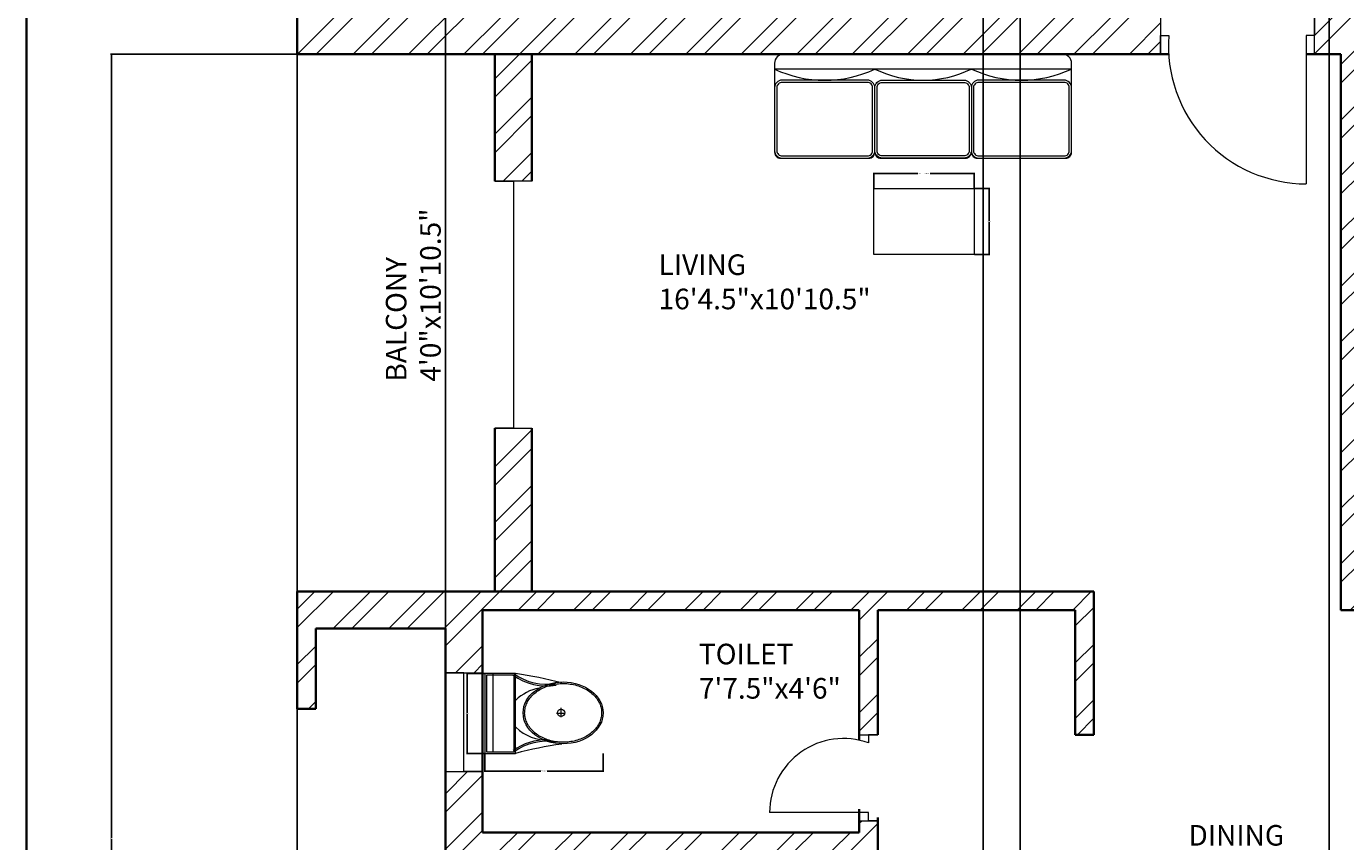
# Model space of a CAD drawing. Units: inches. Extents: x 1513 to 2170, y 1240 to 2288.
# Tile 2 of 10: x 1513 to 1834, y 1603 to 1801. Entities that reach past the tile are written whole.
import ezdxf

# ---------------------------------------------------------------- set-up
doc = ezdxf.new("R2010")
doc.units = ezdxf.units.IN
for name, color, linetype, lineweight in [('A-ANNO-DIMS', 2, 'Continuous', 18), ('A-ANNO-TTLB', 7, 'Continuous', 35), ('A-AREA-IDEN', 7, 'Continuous', 18), ('A-DOOR', 3, 'Continuous', 18), ('A-FLOR-FIXT', 9, 'Continuous', 18), ('A-FLOR-HRAL', 7, 'Continuous', 18), ('A-FURN', 8, 'Continuous', 18), ('A-GLAZ', 4, 'Continuous', 18), ('A-WALL', 7, 'Continuous', 35), ('A-WALL-PATT', 252, 'Continuous', 13)]:
    doc.layers.add(name, color=color, linetype=linetype, lineweight=lineweight)
doc.styles.get("Standard").update_dxf_attribs({"font": 'arial.ttf'})
doc.dimstyles.get("Standard").update_dxf_attribs({"dimtxt": 0.18, "dimasz": 0.18, "dimexe": 0.18, "dimexo": 0.0625, "dimgap": 0.09, "dimtad": 0, "dimtih": 1, "dimtoh": 1, "dimdec": 4, "dimzin": 0, "dimdsep": 46, "dimtxsty": 'Standard', "dimcen": 0.09, "dimadec": 0, "dimazin": 0, "dimtfac": 1, "dimtdec": 4, "dimtofl": 0, "dimtmove": 0, "dimatfit": 3, "dimfxl": 1, "dimtolj": 1, "dimtzin": 0, "dimarcsym": 0})

# ---------------------------------------------------------------- blocks, each defined once
blk = doc.blocks.new('A$C31115884')
for p, q in [((257.5, 466.4), (257.5, 523.2)), ((283.1, 497.7), (223.4, 497.7)), ((0, 200), (0, 0)), ((520, 200), (0, 200)), ((10, 190), (10, 10)), ((510, 190), (10, 190)), ((510, 10), (510, 190)), ((520, 0), (520, 200)), ((510, 54.5), (0, 54.5)), ((10, 10), (510, 10)), ((0, 0), (520, 0))]:
    blk.add_line(p, q)
blk.add_circle((255.6, 496.4), 23.6)
for centre, radius, start, end in [((2777.7, -204.6), 2807, 165.4549, 171.71327), ((-294.5, 403.3), 364.7, 324.20913, 9.34987), ((-294.5, 403.3), 374.7, 324.20913, 9.34987), ((805.8, 403.3), 364.7, 170.65013, 215.79087), ((3237, 905), 2807, 188.28673, 194.5451), ((383.6, 406.2), 293.5, 190.27735, 224.15636), ((139.5, 406.2), 293.5, 315.84364, 2.65635), ((805.8, 403.3), 374.7, 179.20365, 215.79087)]:
    blk.add_arc(centre, radius, start, end)
blk.add_ellipse((256.2, 509.9), major_axis=(0, -260.7), ratio=0.772727)
blk.add_open_spline([(256.2, 259.2), (263.1, 259.2), (270, 259.7), (287.8, 262.3), (298.7, 265.1), (319.9, 273.1), (330.2, 278.4), (350.1, 291.1), (359.7, 298.7), (377.7, 315.9), (386.2, 325.5), (401.7, 346.6), (408.8, 358.1), (421.3, 382.5), (426.8, 395.5), (435.9, 422.4), (439.5, 436.4), (444.8, 465.1), (446.5, 479.7), (447.9, 509.2), (447.6, 524), (445, 553.3), (442.7, 567.8), (436.3, 596), (432.1, 609.7), (421.9, 636), (416, 648.6), (402.5, 672.1), (395, 683), (378.6, 703), (369.8, 712.1), (351.1, 728), (341.3, 734.8), (320.9, 746.2), (310.4, 750.7), (288.9, 757.3), (278, 759.4), (256, 761), (245, 760.6), (223.1, 757.2), (212.3, 754.3), (191.1, 746.1), (180.8, 740.7), (160.9, 727.8), (151.4, 720.1), (133.5, 702.7), (125.1, 693), (109.6, 671.7), (102.6, 660.2), (90.2, 635.7), (84.9, 622.7), (76, 595.6), (72.4, 581.6), (67.2, 552.9), (65.6, 538.2), (64.4, 508.8), (64.8, 494), (67.5, 464.7), (69.9, 450.2), (76.6, 422), (80.8, 408.3), (91.1, 382.2), (97.2, 369.7), (110.8, 346.3), (118.4, 335.4), (134.8, 315.6), (143.7, 306.7), (162.4, 290.9), (172.3, 284.2), (192.8, 273), (203.3, 268.6), (224.8, 262.2), (235.8, 260.2), (249.9, 259.3), (253, 259.2), (256.2, 259.2)], degree=3, knots=[0, 0, 0, 0, 0.110105, 0.110105, 0.285049, 0.285049, 0.459994, 0.459994, 0.634938, 0.634938, 0.809882, 0.809882, 0.984827, 0.984827, 1.159771, 1.159771, 1.334715, 1.334715, 1.50966, 1.50966, 1.684604, 1.684604, 1.859549, 1.859549, 2.034493, 2.034493, 2.209437, 2.209437, 2.384382, 2.384382, 2.559326, 2.559326, 2.73427, 2.73427, 2.909215, 2.909215, 3.084159, 3.084159, 3.259103, 3.259103, 3.434048, 3.434048, 3.608992, 3.608992, 3.783936, 3.783936, 3.958881, 3.958881, 4.133825, 4.133825, 4.30877, 4.30877, 4.483714, 4.483714, 4.658658, 4.658658, 4.833603, 4.833603, 5.008547, 5.008547, 5.183491, 5.183491, 5.358436, 5.358436, 5.53338, 5.53338, 5.708324, 5.708324, 5.883269, 5.883269, 6.058213, 6.058213, 6.233158, 6.233158, 6.283185, 6.283185, 6.283185, 6.283185])
blk = doc.blocks.new('WIN-24')
for p, q in [((0, 24), (9, 24)), ((9, 24), (4.5, 24)), ((4.5, 24), (4.5, 0)), ((4.5, 0), (0, 0)), ((0, 0), (9, 0))]:
    blk.add_line(p, q)
blk = doc.blocks.new('TABLE-COFFEE')
blk.add_lwpolyline([(16.02, 0), (0, 0), (0, 24.35), (16.02, 24.35)], close=True)
blk = doc.blocks.new('*D9')
at = {"layer": 'A-ANNO-DIMS', "color": 0, "lineweight": -2, "transparency": 16777216}
for p, q in [((1624.45, 1624.6), (1624.45, 1620.17)), ((1653.17, 1624.6), (1653.17, 1620.17)), ((1624.63, 1620.35), (1638.03, 1620.35)), ((1652.99, 1620.35), (1639.58, 1620.35))]:
    blk.add_line(p, q, dxfattribs=at)
at = {"layer": 'A-ANNO-DIMS', "color": 0, "transparency": 16777216}
for points in [[(1624.63, 1620.38), (1624.63, 1620.32), (1624.45, 1620.35)], [(1652.99, 1620.38), (1652.99, 1620.32), (1653.17, 1620.35)]]:
    blk.add_solid(points, dxfattribs=at)
at = {"layer": 'Defpoints', "color": 0, "transparency": 16777216}
for p in [(1624.45, 1624.66), (1653.17, 1624.66), (1653.17, 1620.35)]:
    blk.add_point(p, dxfattribs=at)
at = {"layer": 'A-ANNO-DIMS', "color": 0, "transparency": 16777216, "insert": (1638.81, 1620.35), "char_height": 0.18, "attachment_point": 5}
blk.add_mtext('\\A1;WC 29 TYP.', dxfattribs=at)
blk = doc.blocks.new('*D10')
at = {"layer": 'A-ANNO-DIMS', "color": 0, "lineweight": -2, "transparency": 16777216}
for p, q in [((1624.38, 1644.04), (1619.96, 1644.04)), ((1620.14, 1643.86), (1620.14, 1634.53)), ((1620.14, 1624.84), (1620.14, 1634.17)), ((1624.38, 1624.66), (1619.96, 1624.66))]:
    blk.add_line(p, q, dxfattribs=at)
at = {"layer": 'A-ANNO-DIMS', "color": 0, "transparency": 16777216}
for points in [[(1620.11, 1643.86), (1620.17, 1643.86), (1620.14, 1644.04)], [(1620.11, 1624.84), (1620.17, 1624.84), (1620.14, 1624.66)]]:
    blk.add_solid(points, dxfattribs=at)
at = {"layer": 'Defpoints', "color": 0, "transparency": 16777216}
for p in [(1624.45, 1644.04), (1620.14, 1624.66), (1624.45, 1624.66)]:
    blk.add_point(p, dxfattribs=at)
at = {"layer": 'A-ANNO-DIMS', "color": 0, "transparency": 16777216, "insert": (1620.14, 1634.35), "char_height": 0.18, "attachment_point": 5}
blk.add_mtext('\\A1;19 TYP.', dxfattribs=at)
blk = doc.blocks.new('*D23')
at = {"layer": 'A-ANNO-DIMS', "color": 0, "lineweight": -2, "transparency": 16777216}
for p, q in [((1718.92, 1761.92), (1718.92, 1765.69)), ((1719.1, 1765.51), (1729.59, 1765.51)), ((1743.09, 1765.51), (1732.6, 1765.51)), ((1743.27, 1761.92), (1743.27, 1765.69))]:
    blk.add_line(p, q, dxfattribs=at)
at = {"layer": 'A-ANNO-DIMS', "color": 0, "transparency": 16777216}
for points in [[(1719.1, 1765.54), (1719.1, 1765.48), (1718.92, 1765.51)], [(1743.09, 1765.54), (1743.09, 1765.48), (1743.27, 1765.51)]]:
    blk.add_solid(points, dxfattribs=at)
at = {"layer": 'Defpoints', "color": 0, "transparency": 16777216}
for p in [(1718.92, 1765.51), (1718.92, 1761.86), (1743.27, 1761.86)]:
    blk.add_point(p, dxfattribs=at)
at = {"layer": 'A-ANNO-DIMS', "color": 0, "transparency": 16777216, "insert": (1731.1, 1765.51), "char_height": 0.18, "attachment_point": 5}
blk.add_mtext('\\A1;COFFEE TABLE 24 TYP.', dxfattribs=at)
blk = doc.blocks.new('*D24')
at = {"layer": 'A-ANNO-DIMS', "color": 0, "lineweight": -2, "transparency": 16777216}
for p, q in [((1743.34, 1761.86), (1747.11, 1761.86)), ((1746.93, 1761.68), (1746.93, 1754.03)), ((1746.93, 1746.02), (1746.93, 1753.67)), ((1743.34, 1745.84), (1747.11, 1745.84))]:
    blk.add_line(p, q, dxfattribs=at)
at = {"layer": 'A-ANNO-DIMS', "color": 0, "transparency": 16777216}
for points in [[(1746.9, 1761.68), (1746.96, 1761.68), (1746.93, 1761.86)], [(1746.9, 1746.02), (1746.96, 1746.02), (1746.93, 1745.84)]]:
    blk.add_solid(points, dxfattribs=at)
at = {"layer": 'Defpoints', "color": 0, "transparency": 16777216}
for p in [(1743.27, 1761.86), (1746.93, 1761.86), (1743.27, 1745.84)]:
    blk.add_point(p, dxfattribs=at)
at = {"layer": 'A-ANNO-DIMS', "color": 0, "transparency": 16777216, "insert": (1746.93, 1753.85), "char_height": 0.18, "attachment_point": 5}
blk.add_mtext('\\A1;16 TYP.', dxfattribs=at)
blk = doc.blocks.new('*D27')
at = {"layer": 'A-ANNO-DIMS', "color": 0, "lineweight": -2, "transparency": 16777216}
for p, q in [((1578.87, 1956.42), (1578.87, 1344.15)), ((1614.87, 1956.42), (1614.87, 1344.15)), ((1579.05, 1344.33), (1596.65, 1344.33)), ((1614.69, 1344.33), (1597.08, 1344.33))]:
    blk.add_line(p, q, dxfattribs=at)
at = {"layer": 'A-ANNO-DIMS', "color": 0, "transparency": 16777216}
for points in [[(1579.05, 1344.36), (1579.05, 1344.3), (1578.87, 1344.33)], [(1614.69, 1344.36), (1614.69, 1344.3), (1614.87, 1344.33)]]:
    blk.add_solid(points, dxfattribs=at)
at = {"layer": 'Defpoints', "color": 0, "transparency": 16777216}
for p in [(1578.87, 1956.48), (1614.87, 1956.48), (1614.87, 1344.33)]:
    blk.add_point(p, dxfattribs=at)
at = {"layer": 'A-ANNO-DIMS', "color": 0, "transparency": 16777216, "insert": (1596.87, 1344.33), "char_height": 0.18, "attachment_point": 5}
blk.add_mtext('\\A1;36', dxfattribs=at)
blk = doc.blocks.new('*D29')
at = {"layer": 'A-ANNO-DIMS', "color": 0, "lineweight": -2, "transparency": 16777216}
for p, q in [((1578.8, 1794.48), (1533.54, 1794.48)), ((1533.72, 1794.3), (1533.72, 1604.16)), ((1533.72, 1413.66), (1533.72, 1603.8)), ((1614.8, 1413.48), (1533.54, 1413.48))]:
    blk.add_line(p, q, dxfattribs=at)
at = {"layer": 'A-ANNO-DIMS', "color": 0, "transparency": 16777216}
for points in [[(1533.69, 1794.3), (1533.75, 1794.3), (1533.72, 1794.48)], [(1533.69, 1413.66), (1533.75, 1413.66), (1533.72, 1413.48)]]:
    blk.add_solid(points, dxfattribs=at)
at = {"layer": 'Defpoints', "color": 0, "transparency": 16777216}
for p in [(1533.72, 1794.48), (1578.87, 1794.48), (1614.87, 1413.48)]:
    blk.add_point(p, dxfattribs=at)
at = {"layer": 'A-ANNO-DIMS', "color": 0, "transparency": 16777216, "insert": (1533.72, 1603.98), "char_height": 0.18, "attachment_point": 5}
blk.add_mtext('\\A1;381', dxfattribs=at)
blk = doc.blocks.new('*D34')
at = {"layer": 'A-ANNO-DIMS', "color": 0, "lineweight": -2, "transparency": 16777216}
for p, q in [((1745.46, 1803.42), (1745.46, 1344.15)), ((1754.46, 1803.42), (1754.46, 1344.15)), ((1745.64, 1344.33), (1749.81, 1344.33)), ((1754.28, 1344.33), (1750.11, 1344.33))]:
    blk.add_line(p, q, dxfattribs=at)
at = {"layer": 'A-ANNO-DIMS', "color": 0, "transparency": 16777216}
for points in [[(1745.64, 1344.36), (1745.64, 1344.3), (1745.46, 1344.33)], [(1754.28, 1344.36), (1754.28, 1344.3), (1754.46, 1344.33)]]:
    blk.add_solid(points, dxfattribs=at)
at = {"layer": 'Defpoints', "color": 0, "transparency": 16777216}
for p in [(1745.46, 1803.48), (1754.46, 1803.48), (1754.46, 1344.33)]:
    blk.add_point(p, dxfattribs=at)
at = {"layer": 'A-ANNO-DIMS', "color": 0, "transparency": 16777216, "insert": (1749.96, 1344.33), "char_height": 0.18, "attachment_point": 5}
blk.add_mtext('\\A1;9', dxfattribs=at)
blk = doc.blocks.new('*D36')
at = {"layer": 'A-ANNO-DIMS', "color": 0, "lineweight": -2, "transparency": 16777216}
for p, q in [((1829.49, 1887.42), (1829.49, 1344.15)), ((1864.51, 1887.42), (1864.51, 1344.15)), ((1829.67, 1344.33), (1846.61, 1344.33)), ((1864.33, 1344.33), (1847.39, 1344.33))]:
    blk.add_line(p, q, dxfattribs=at)
at = {"layer": 'A-ANNO-DIMS', "color": 0, "transparency": 16777216}
for points in [[(1829.67, 1344.36), (1829.67, 1344.3), (1829.49, 1344.33)], [(1864.33, 1344.36), (1864.33, 1344.3), (1864.51, 1344.33)]]:
    blk.add_solid(points, dxfattribs=at)
at = {"layer": 'Defpoints', "color": 0, "transparency": 16777216}
for p in [(1829.49, 1887.48), (1864.51, 1887.48), (1864.51, 1344.33)]:
    blk.add_point(p, dxfattribs=at)
at = {"layer": 'A-ANNO-DIMS', "color": 0, "transparency": 16777216, "insert": (1847, 1344.33), "char_height": 0.18, "attachment_point": 5}
blk.add_mtext('\\A1;35.02', dxfattribs=at)

msp = doc.modelspace()

# ---------------------------------------------------------------- hatches: boundary and pattern name
at = {"layer": 'A-WALL-PATT'}
h = msp.add_hatch(dxfattribs=at)
h.set_pattern_fill('ANSI32', color=256)
h.paths.add_polyline_path([(2041.852, 1719.48), (2014.852, 1719.48), (2014.852, 1734.444), (2005.852, 1734.444), (2005.852, 1710.48), (2032.852, 1710.48), (2032.852, 1663.98), (1976.619, 1663.98), (1976.619, 1659.48), (2005.852, 1659.48), (2005.852, 1626.27), (2014.852, 1626.27), (2014.852, 1659.48), (2041.852, 1659.48)])
h.paths.add_polyline_path([(1954.521, 1663.98), (1875.357, 1663.98), (1875.357, 1659.48), (1945.852, 1659.48), (1945.852, 1546.98), (1950.352, 1546.98), (2005.852, 1546.98), (2005.852, 1422.48), (1985.47, 1422.48), (1985.47, 1413.48), (2014.852, 1413.48), (2014.852, 1602.27), (2005.852, 1602.27), (2005.852, 1551.48), (1950.352, 1551.48), (1950.352, 1659.48), (1954.521, 1659.48)])
h.paths.add_polyline_path([(1949.47, 1422.48), (1937.366, 1422.48), (1937.366, 1413.48), (1949.47, 1413.48)], flags=0)
h.paths.add_polyline_path([(1937.366, 1422.48), (1908.866, 1422.48), (1908.866, 1546.98), (1805.486, 1546.98), (1805.486, 1542.48), (1904.366, 1542.48), (1904.366, 1451.2), (1897.222, 1451.2), (1897.222, 1442.2), (1904.366, 1442.2), (1904.366, 1422.48), (1904.366, 1413.48), (1904.366, 1389.48), (1908.866, 1389.48), (1908.866, 1413.48), (1932.866, 1413.48), (1932.866, 1389.48), (1937.366, 1389.48)])
h.paths.add_polyline_path([(1830.254, 1442.2), (1844.144, 1442.2), (1844.144, 1451.2), (1830.254, 1451.2), (1821.254, 1451.2), (1821.254, 1422.48), (1766.366, 1422.48), (1766.366, 1542.48), (1770.265, 1542.48), (1770.265, 1546.98), (1758.774, 1546.98), (1758.774, 1544.73), (1758.774, 1542.48), (1761.866, 1542.48), (1761.866, 1389.48), (1779.454, 1389.48), (1779.454, 1398.48), (1770.866, 1398.48), (1770.866, 1413.48), (1830.254, 1413.48)])
h.paths.add_polyline_path([(1686.156, 1451.2), (1677.156, 1451.2), (1677.156, 1422.48), (1623.866, 1422.48), (1623.866, 1460.073), (1614.866, 1460.073), (1614.866, 1413.48), (1686.156, 1413.48)])
h.paths.add_polyline_path([(1761.866, 1422.48), (1686.156, 1422.48), (1686.156, 1413.48), (1761.866, 1413.48)])
h.paths.add_polyline_path([(1623.866, 1542.48), (1688.266, 1542.48), (1688.266, 1544.73), (1688.266, 1546.98), (1623.866, 1546.98), (1623.866, 1560.442), (1614.866, 1560.442), (1614.866, 1520.073), (1619.366, 1520.073), (1623.866, 1520.073)])
h.paths.add_polyline_path([(1623.866, 1600.98), (1715.366, 1600.98), (1715.366, 1546.98), (1711.055, 1546.98), (1711.055, 1542.48), (1719.866, 1542.48), (1726.867, 1542.48), (1726.867, 1544.73), (1726.867, 1546.98), (1719.866, 1546.98), (1719.866, 1600.98), (1719.866, 1608.301), (1717.616, 1608.301), (1715.366, 1608.301), (1715.366, 1605.48), (1623.866, 1605.48), (1623.866, 1620.254), (1614.866, 1620.254), (1614.866, 1584.442), (1623.866, 1584.442)])
h.paths.add_polyline_path([(1623.866, 1659.48), (1715.366, 1659.48), (1715.366, 1629.2), (1719.866, 1629.2), (1719.866, 1659.48), (1767.866, 1659.48), (1767.866, 1629.2), (1772.366, 1629.2), (1772.366, 1663.98), (1578.866, 1663.98), (1578.866, 1661.73), (1578.866, 1659.48), (1578.866, 1635.48), (1583.366, 1635.48), (1583.366, 1654.98), (1614.866, 1654.98), (1614.866, 1644.254), (1619.366, 1644.254), (1623.866, 1644.254)])
h.paths.add_polyline_path([(1788.587, 1798.98), (1788.587, 1803.48), (1623.866, 1803.48), (1623.866, 1887.48), (1829.49, 1887.48), (1829.49, 1891.98), (1829.49, 1896.48), (1748.366, 1896.48), (1743.866, 1896.48), (1623.866, 1896.48), (1623.866, 1904.333), (1619.366, 1904.333), (1614.866, 1904.333), (1614.866, 1896.48), (1578.866, 1896.48), (1578.866, 1887.48), (1614.866, 1887.48), (1614.866, 1803.48), (1578.866, 1803.48), (1578.866, 1794.48), (1626.866, 1794.48), (1788.587, 1794.48)])
h.paths.add_polyline_path([(1635.866, 1794.48), (1626.866, 1794.48), (1626.866, 1763.627), (1631.366, 1763.627), (1635.866, 1763.627)])
h.paths.add_polyline_path([(1635.866, 1703.627), (1626.866, 1703.627), (1626.866, 1663.98), (1635.866, 1663.98)])
h.paths.add_polyline_path([(1587.866, 2016.48), (1614.866, 2016.48), (1623.866, 2016.48), (1707.767, 2016.48), (1707.767, 2018.73), (1707.767, 2020.98), (1706.366, 2020.98), (1706.366, 2025.944), (1701.866, 2025.944), (1701.866, 2020.98), (1623.866, 2020.98), (1623.866, 2045.903), (1614.866, 2045.903), (1614.866, 2025.48), (1583.366, 2025.48), (1583.366, 2040.48), (1578.866, 2040.48), (1578.866, 2016.48), (1578.866, 1956.48), (1614.866, 1956.48), (1614.866, 1946.333), (1623.866, 1946.333), (1623.866, 1965.48), (1587.866, 1965.48)])
h.paths.add_polyline_path([(1748.366, 2016.48), (1748.366, 2025.48), (1743.866, 2025.48), (1739.366, 2025.48), (1739.366, 2020.98), (1738.09, 2020.98), (1738.09, 2016.48), (1743.866, 2016.48), (1743.866, 1896.48), (1748.366, 1896.48)])
h.paths.add_polyline_path([(1746.736, 2085.48), (1623.866, 2085.48), (1623.866, 2205.48), (1657.136, 2205.48), (1657.136, 2214.48), (1614.866, 2214.48), (1614.866, 2069.903), (1623.866, 2069.903), (1623.866, 2080.98), (1683.866, 2080.98), (1701.866, 2080.98), (1701.866, 2046.743), (1706.366, 2046.743), (1706.366, 2080.98), (1746.736, 2080.98)])
h = msp.add_hatch(dxfattribs=at)
h.set_pattern_fill('ANSI32', color=256)
h.paths.add_polyline_path([(1744.852, 2209.98), (1762.042, 2209.98), (1762.042, 2214.48), (1715.345, 2214.48), (1715.345, 2205.48), (1735.852, 2205.48), (1735.852, 2161.98), (1733.253, 2161.98), (1719.866, 2161.98), (1719.866, 2112.429), (1724.366, 2112.429), (1724.366, 2152.98), (1762.042, 2152.98), (1870.852, 2152.98), (1870.852, 2080.98), (1875.352, 2080.98), (1878.245, 2080.98), (1878.245, 2083.23), (1878.245, 2085.48), (1875.352, 2085.48), (1875.352, 2173.929), (1881.628, 2173.929), (1881.628, 2178.429), (1881.628, 2182.929), (1875.352, 2182.929), (1875.352, 2214.48), (1858.335, 2214.48), (1858.335, 2209.98), (1866.352, 2209.98), (1866.352, 2161.98), (1762.042, 2161.98), (1744.852, 2161.98)])
h.paths.add_polyline_path([(2014.852, 2214.48), (1944.011, 2214.48), (1944.011, 2182.929), (1938.347, 2182.929), (1938.347, 2173.929), (1953.011, 2173.929), (1953.011, 2182.929), (1953.011, 2205.48), (2005.852, 2205.48), (2005.852, 2085.48), (1955.061, 2085.48), (1955.061, 2080.98), (2005.852, 2080.98), (2005.852, 2068.903), (2014.852, 2068.903)])
h.paths.add_polyline_path([(2014.852, 2044.903), (2005.852, 2044.903), (2005.852, 2020.98), (1926.352, 2020.98), (1926.352, 2080.98), (1930.882, 2080.98), (1930.882, 2083.23), (1930.882, 2085.48), (1921.852, 2085.48), (1915.536, 2085.48), (1915.536, 2083.23), (1915.536, 2080.98), (1921.852, 2080.98), (1921.852, 2020.98), (1916.378, 2020.98), (1916.378, 2018.73), (1916.378, 2016.48), (2005.852, 2016.48), (2005.852, 2009.442), (2014.852, 2009.442), (2014.852, 2016.48), (2029.852, 2016.48), (2041.852, 2016.48), (2041.852, 2040.48), (2037.352, 2040.48), (2037.352, 2036.595), (2037.352, 2020.98), (2014.852, 2020.98)])
h.paths.add_polyline_path([(2041.852, 1956.48), (2014.852, 1956.48), (2014.852, 1963.797), (2005.852, 1963.797), (2005.852, 1947.48), (2032.852, 1947.48), (2032.852, 1896.48), (1978.852, 1896.48), (1978.852, 1891.98), (1978.852, 1887.48), (2005.852, 1887.48), (2005.852, 1862.401), (2014.852, 1862.401), (2014.852, 1887.48), (2037.352, 1887.48), (2037.352, 1863.48), (2041.852, 1863.48), (2041.852, 1887.48), (2041.852, 1896.48)], flags=17)
h.paths.add_polyline_path([(1885.852, 1896.48), (1885.852, 1920.48), (1878.866, 1920.48), (1878.866, 2016.48), (1881.925, 2016.48), (1881.925, 2018.73), (1881.925, 2020.98), (1874.366, 2020.98), (1874.366, 1896.48), (1864.508, 1896.48), (1864.508, 1887.48), (1876.852, 1887.48), (1876.852, 1855.773), (1885.852, 1855.773), (1885.852, 1868.947), (1942.852, 1868.947), (1942.852, 1803.48), (1885.852, 1803.48), (1885.852, 1817.861), (1876.852, 1817.861), (1876.852, 1803.48), (1825.976, 1803.48), (1825.976, 1798.98), (1825.976, 1794.48), (1832.366, 1794.48), (1832.366, 1663.98), (1832.366, 1659.48), (1841.939, 1659.48), (1841.939, 1661.73), (1841.939, 1663.98), (1836.866, 1663.98), (1836.866, 1794.48), (1992.866, 1794.48), (2005.852, 1794.48), (2005.852, 1784.304), (2010.352, 1784.304), (2014.852, 1784.304), (2014.852, 1794.48), (2041.852, 1794.48), (2041.852, 1803.48), (2014.852, 1803.48), (2014.852, 1838.401), (2005.852, 1838.401), (2005.852, 1803.48), (1951.852, 1803.48), (1951.852, 1887.48), (1956.114, 1887.48), (1956.114, 1891.98), (1956.114, 1896.48), (1951.852, 1896.48), (1951.852, 1920.48), (1947.352, 1920.48), (1947.352, 1896.48), (1942.852, 1896.48), (1942.852, 1877.947), (1885.852, 1877.947)])

# ---------------------------------------------------------------- linework, layer by layer
at = {"layer": 'A-ANNO-TTLB'}
msp.add_lwpolyline([(1513.071, 2287.731), (2170.435, 2287.731), (2170.435, 1239.669), (1513.071, 1239.669)], close=True, dxfattribs=at)
at = {"layer": 'A-DOOR'}
for p, q in [((1788.587, 1803.48), (1788.587, 1794.48)), ((1825.976, 1794.48), (1825.976, 1803.48)), ((1825.976, 1803.48), (1825.976, 1798.98)), ((1788.587, 1794.48), (1788.587, 1798.98)), ((1788.587, 1798.98), (1790.587, 1798.98)), ((1825.976, 1798.98), (1823.976, 1798.98)), ((1823.976, 1798.98), (1823.976, 1762.98)), ((1635.866, 1763.627), (1626.866, 1763.627)), ((1626.866, 1763.627), (1631.366, 1763.627)), ((1631.366, 1763.627), (1631.366, 1703.627)), ((1631.366, 1703.627), (1626.866, 1703.627)), ((1626.866, 1703.627), (1635.866, 1703.627)), ((1715.366, 1629.2), (1719.866, 1629.2)), ((1719.866, 1629.2), (1717.616, 1629.2)), ((1717.616, 1629.2), (1717.616, 1627.2)), ((1717.616, 1610.301), (1693.616, 1610.301)), ((1717.616, 1608.301), (1717.616, 1610.301)), ((1715.366, 1608.301), (1719.866, 1608.301)), ((1719.866, 1608.301), (1717.616, 1608.301))]:
    msp.add_line(p, q, dxfattribs=at)
for centre, radius, start, end in [((1823.976, 1796.463), 33.483, 175.68974, 270), ((1711.565, 1610.301), 17.949, 70.29874, 180)]:
    msp.add_arc(centre, radius, start, end, dxfattribs=at)
at = {"layer": 'A-FLOR-HRAL'}
msp.add_line((1578.866, 1794.48), (1578.866, 1661.73), dxfattribs=at)
at = {"layer": 'A-FURN', "ltscale": 0.03}
msp.add_lwpolyline([(1744.068, 1769.233), (1765.51, 1769.233, 0.4142136), (1766.953, 1770.676), (1766.953, 1792.316, 0.4142136), (1764.789, 1794.48), (1696.984, 1794.48, 0.4142136), (1694.82, 1792.316), (1694.82, 1770.676, 0.4142136), (1696.263, 1769.233), (1717.704, 1769.233, 0.4142136), (1719.147, 1770.676, -1), (1719.183, 1770.676, 0.4142136), (1720.625, 1769.233), (1741.148, 1769.233, 0.4142136), (1742.59, 1770.676, -1), (1742.626, 1770.676, 0.4142136)], format="xyb", close=True, dxfattribs=at)
at = {"layer": 'A-FURN'}
msp.add_lwpolyline([(1766.953, 1790.873), (1694.82, 1790.873)], dxfattribs=at)
for points in [[(1719.165, 1771.036), (1719.165, 1786.365, 0.4142136), (1717.361, 1788.168), (1696.623, 1788.168, 0.4142136), (1694.82, 1786.365), (1694.82, 1771.036, 0.4142136), (1696.623, 1769.233), (1717.361, 1769.233, 0.4142136)], [(1719.165, 1771.036), (1719.165, 1786.365, -0.4142136), (1720.968, 1788.168), (1740.805, 1788.168, -0.4142136), (1742.608, 1786.365), (1742.608, 1771.036, -0.4142136), (1740.805, 1769.233), (1720.968, 1769.233, -0.4142136)], [(1766.953, 1771.036), (1766.953, 1786.365, 0.4142136), (1765.149, 1788.168), (1744.411, 1788.168, 0.4142136), (1742.608, 1786.365), (1742.608, 1771.036, 0.4142136), (1744.411, 1769.233), (1765.149, 1769.233, 0.4142136)], [(1718.624, 1771.036), (1718.624, 1786.365, 0.4142136), (1717.361, 1787.627), (1696.623, 1787.627, 0.4142136), (1695.361, 1786.365), (1695.361, 1771.036, 0.4142136), (1696.623, 1769.774), (1717.361, 1769.774, 0.4142136)], [(1719.706, 1771.036), (1719.706, 1786.365, -0.4142136), (1720.968, 1787.627), (1740.805, 1787.627, -0.4142136), (1742.067, 1786.365), (1742.067, 1771.036, -0.4142136), (1740.805, 1769.774), (1720.968, 1769.774, -0.4142136)], [(1766.412, 1771.036), (1766.412, 1786.365, 0.4142136), (1765.149, 1787.627), (1744.411, 1787.627, 0.4142136), (1743.149, 1786.365), (1743.149, 1771.036, 0.4142136), (1744.411, 1769.774), (1765.149, 1769.774, 0.4142136)]]:
    msp.add_lwpolyline(points, format="xyb", close=True, dxfattribs=at)
for centre, radius, start, end in [((1706.992, 1816.57), 28.434, 244.65382, 295.34618), ((1730.886, 1814.767), 26.614, 243.869, 296.131), ((1754.78, 1816.871), 28.706, 244.91063, 295.08937)]:
    msp.add_arc(centre, radius, start, end, dxfattribs=at)
at = {"layer": 'A-WALL'}
for p, q in [((1578.866, 1803.48), (1578.866, 1794.48)), ((1578.866, 1794.48), (1790.551, 1794.48)), ((1578.866, 1794.48), (1626.866, 1794.48)), ((1626.866, 1794.48), (1626.866, 1763.627)), ((1635.866, 1794.48), (1790.551, 1794.48)), ((1635.866, 1763.627), (1635.866, 1794.48)), ((1823.976, 1794.48), (1832.366, 1794.48)), ((1823.976, 1794.48), (1832.366, 1794.48)), ((1832.366, 1794.48), (1832.366, 1663.98)), ((1626.866, 1703.627), (1626.866, 1663.98)), ((1635.866, 1663.98), (1635.866, 1703.627)), ((1578.866, 1663.98), (1772.366, 1663.98)), ((1578.866, 1663.98), (1578.866, 1659.48)), ((1626.866, 1663.98), (1635.866, 1663.98)), ((1772.366, 1629.2), (1772.366, 1663.98)), ((1832.366, 1663.98), (1832.366, 1659.48)), ((1578.866, 1659.48), (1578.866, 1635.48)), ((1623.866, 1659.48), (1623.866, 1605.48)), ((1623.866, 1659.48), (1715.366, 1659.48)), ((1715.366, 1627.843), (1715.366, 1659.48)), ((1719.866, 1629.2), (1719.866, 1659.48)), ((1719.866, 1659.48), (1767.866, 1659.48)), ((1719.866, 1659.48), (1767.866, 1659.48)), ((1767.866, 1659.48), (1767.866, 1629.2)), ((1832.366, 1659.48), (1841.939, 1659.48)), ((1583.366, 1635.48), (1583.366, 1654.98)), ((1614.866, 1654.98), (1583.366, 1654.98)), ((1614.866, 1654.98), (1614.866, 1413.48)), ((1578.866, 1635.48), (1583.366, 1635.48)), ((1767.866, 1629.2), (1772.366, 1629.2)), ((1715.366, 1611.123), (1715.366, 1605.48)), ((1719.866, 1600.98), (1719.866, 1609.123)), ((1715.366, 1605.48), (1623.866, 1605.48))]:
    msp.add_line(p, q, dxfattribs=at)

# ---------------------------------------------------------------- block references
at = {"layer": 'A-FLOR-FIXT', "xscale": 0.0372717239612423, "yscale": 0.0372717239612423, "zscale": 0.0372717239612423, "rotation": 270}
msp.add_blockref('A$C31115884', (1624.447, 1644.042), dxfattribs=at)
at = {"layer": 'A-FURN', "rotation": 90}
msp.add_blockref('TABLE-COFFEE', (1743.274, 1745.84), dxfattribs=at)
at = {"layer": 'A-GLAZ', "extrusion": (0, 0, -1), "zscale": -1, "rotation": 180}
msp.add_blockref('WIN-24', (-1614.863, 1644.255), dxfattribs=at)

# ---------------------------------------------------------------- texts
at = {"layer": 'A-AREA-IDEN', "insert": (1600.39, 1714.945), "char_height": 5, "attachment_point": 1, "rotation": 90}
msp.add_mtext_dynamic_manual_height_columns('BALCONY\\P4\'0"x10\'10.5"', width=92.69084, gutter_width=12.5, heights=[0], dxfattribs=at)
at = {"layer": 'A-AREA-IDEN', "char_height": 5, "attachment_point": 1}
for s, width, insert in [('LIVING\\P16\'4.5"x10\'10.5"', 224.44512, (1666.636, 1745.853)), ('TOILET\\P7\'7.5"x4\'6"', 127.98283, (1676.43, 1651.289)), ('DINING\\P17\'9"x9\'0"', 261.8017, (1795.355, 1607.258))]:
    msp.add_mtext_dynamic_manual_height_columns(s, width=width, gutter_width=12.5, heights=[0], dxfattribs=dict(at, insert=insert))

# ---------------------------------------------------------------- dimensions: what is measured, and where the dimension line sits
at = {"layer": 'A-ANNO-DIMS'}
for base, p1, p2, override, picture, middle in [((1614.866, 1344.33), (1578.866, 1956.48), (1614.866, 1956.48), {"dimdec": 0, "dimlfac": 1, "dimrnd": 0, "dimzin": 0, "dimdsep": 46, "dimlunit": 2}, '*D27', (1596.866, 1344.33)), ((1864.508, 1344.33), (1829.49, 1887.48), (1864.508, 1887.48), {"dimdec": 2, "dimlfac": 1, "dimrnd": 0, "dimzin": 0, "dimdsep": 46, "dimlunit": 2}, '*D36', (1846.999, 1344.33)), ((1754.464, 1344.33), (1745.464, 1803.48), (1754.464, 1803.48), {"dimdec": 0, "dimlfac": 1, "dimrnd": 0, "dimzin": 0, "dimdsep": 46, "dimlunit": 2}, '*D34', (1749.964, 1344.33))]:
    dim = msp.add_linear_dim(base=base, p1=p1, p2=p2, dimstyle='Standard', override=override, dxfattribs=at)
    dim.commit()
    dim.dimension.update_dxf_attribs({"geometry": picture, "text_midpoint": middle})
dim = msp.add_linear_dim(base=(1533.716, 1794.48), p1=(1614.866, 1413.48), p2=(1578.866, 1794.48), angle=90, dimstyle='Standard', override={"dimdec": 0, "dimlfac": 1, "dimrnd": 0, "dimzin": 0, "dimdsep": 46, "dimlunit": 2}, dxfattribs=at)
dim.commit()
dim.dimension.update_dxf_attribs({"geometry": '*D29', "text_midpoint": (1533.716, 1603.98)})
for base, p1, p2, angle, text, picture, middle in [((1718.923, 1765.511), (1743.273, 1761.859), (1718.923, 1761.859), 180, 'COFFEE TABLE <> TYP.', '*D23', (1731.098, 1765.511)), ((1746.925, 1761.859), (1743.273, 1745.836), (1743.273, 1761.859), 90, '<> TYP.', '*D24', (1746.925, 1753.847)), ((1620.139, 1624.66), (1624.447, 1644.042), (1624.447, 1624.66), 270, '<> TYP.', '*D10', (1620.139, 1634.351))]:
    dim = msp.add_linear_dim(base=base, p1=p1, p2=p2, angle=angle, text=text, dimstyle='Standard', override={"dimdec": 0, "dimlfac": 1, "dimrnd": 0, "dimzin": 0, "dimdsep": 46, "dimlunit": 2}, dxfattribs=at)
    dim.commit()
    dim.dimension.update_dxf_attribs({"geometry": picture, "text_midpoint": middle})
dim = msp.add_linear_dim(base=(1653.167, 1620.352), p1=(1624.447, 1624.66), p2=(1653.167, 1624.66), text='WC <> TYP.', dimstyle='Standard', override={"dimdec": 0, "dimlfac": 1, "dimrnd": 0, "dimzin": 0, "dimdsep": 46, "dimlunit": 2}, dxfattribs=at)
dim.commit()
dim.dimension.update_dxf_attribs({"geometry": '*D9', "text_midpoint": (1638.807, 1620.352)})

doc.saveas('drawing.dxf')
